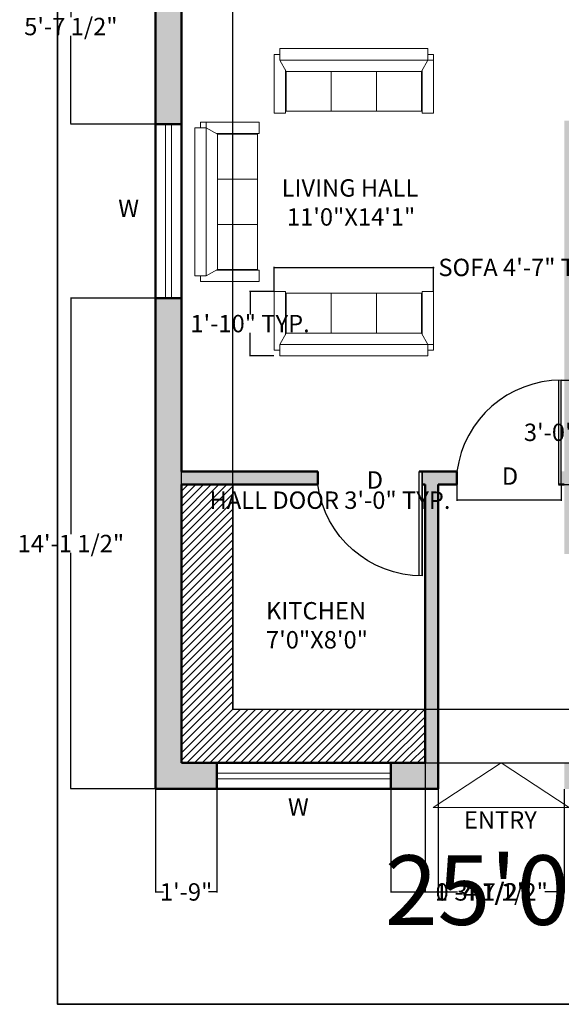
# Model space of a CAD drawing. Units: inches. Extents: x 125920 to 126336, y 366134 to 366735.
# Tile 1 of 6: x 125920 to 126106, y 366134 to 366473. Entities that reach past the tile are written whole.
import ezdxf

# ---------------------------------------------------------------- set-up
doc = ezdxf.new("R2010")
doc.units = ezdxf.units.IN
doc.header["$MEASUREMENT"] = 0
for name, color, linetype, lineweight in [('A-ANNO-DIMS', 2, 'Continuous', 18), ('A-ANNO-SYMB', 7, 'Continuous', 18), ('A-ANNO-TEXT', 7, 'Continuous', 18), ('A-ANNO-TTLB', 7, 'Continuous', 35), ('A-AREA-IDEN', 7, 'Continuous', 25), ('A-DOOR', 3, 'Continuous', 25), ('A-FLOR-FIXT', 8, 'Continuous', 25), ('A-FLOR-FIXT-PATT', 7, 'Continuous', 13), ('A-FURN', 8, 'Continuous', 18), ('A-GLAZ', 4, 'Continuous', 18), ('A-WALL', 7, 'Continuous', 50)]:
    doc.layers.add(name, color=color, linetype=linetype, lineweight=lineweight)
doc.layers.add('A-WALL-PATT', color=18, linetype='Continuous', lineweight=13, true_color=0x000000)
doc.styles.get("Standard").update_dxf_attribs({"font": 'arial.ttf'})
doc.dimstyles.get("Standard").update_dxf_attribs({"dimtxt": 6, "dimasz": 0.18, "dimexe": 0.18, "dimexo": 0.0625, "dimgap": 0.09, "dimtad": 0, "dimtih": 1, "dimtoh": 1, "dimdec": 1, "dimzin": 0, "dimdsep": 46, "dimlunit": 3, "dimtxsty": 'Standard', "dimcen": 0.09, "dimadec": 0, "dimazin": 0, "dimtfac": 1, "dimtdec": 1, "dimtofl": 0, "dimtmove": 0, "dimatfit": 3, "dimfxl": 1, "dimtolj": 1, "dimtzin": 0, "dimarcsym": 0})

# ---------------------------------------------------------------- blocks, each defined once
blk = doc.blocks.new('SOFA-3-SEAT')
for p, q in [((1.96, 55.04), (22.23, 55.04)), ((1.96, 55.04), (1.96, 53.08)), ((3.92, 55.04), (3.92, 1.96)), ((22.23, 51.12), (22.23, 55.04)), ((0, 53.08), (0, 1.96)), ((3.92, 53.08), (0, 53.08)), ((3.92, 53.08), (7.85, 50.88)), ((7.54, 51.12), (22.23, 51.12)), ((21.58, 50.87), (7.85, 50.87)), ((21.58, 35.3), (7.85, 35.3)), ((21.58, 19.74), (7.85, 19.74)), ((7.85, 4.17), (3.92, 1.96)), ((7.29, 3.92), (22.23, 3.92)), ((22.23, 3.92), (22.23, 0)), ((3.92, 1.96), (0, 1.96)), ((1.96, 1.96), (1.96, 0)), ((1.96, 0), (22.23, 0))]:
    blk.add_line(p, q)
blk.add_lwpolyline([(7.85, 50.88), (7.85, 4.17), (21.58, 4.17), (21.58, 50.87)])
blk = doc.blocks.new('WIN-60')
for p, q in [((0, 0), (0, 60)), ((3.5, 0), (3.5, 60)), ((5.5, 60), (5.5, 0)), ((9, 60), (9, 0))]:
    blk.add_line(p, q)
blk = doc.blocks.new('DOOR-36-WALL-4_5')
for p, q in [((0, 36), (0, 0)), ((0, 36), (1, 36)), ((1, 0), (1, 36))]:
    blk.add_line(p, q)
blk.add_arc((0, 36.32), 36.32, 270, 352.3719)
blk = doc.blocks.new('*D21')
at = {"layer": 'A-ANNO-DIMS', "color": 0, "lineweight": -2, "transparency": 16777216}
for p, q in [((126007.38, 366379.47), (126007.38, 366387.84)), ((126007.56, 366387.66), (126062.24, 366387.66)), ((126062.42, 366379.47), (126062.42, 366387.84)), ((126062.42, 366387.66), (126062.6, 366387.66))]:
    blk.add_line(p, q, dxfattribs=at)
at = {"layer": 'A-ANNO-DIMS', "color": 0, "transparency": 16777216}
for points in [[(126007.56, 366387.69), (126007.56, 366387.63), (126007.38, 366387.66)], [(126062.24, 366387.69), (126062.24, 366387.63), (126062.42, 366387.66)]]:
    blk.add_solid(points, dxfattribs=at)
at = {"layer": 'Defpoints', "color": 0, "transparency": 16777216}
for p in [(126062.42, 366387.66), (126007.38, 366379.4), (126062.42, 366379.4)]:
    blk.add_point(p, dxfattribs=at)
at = {"layer": 'A-ANNO-DIMS', "color": 0, "transparency": 16777216, "insert": (126093.54, 366387.66), "char_height": 6, "attachment_point": 5}
blk.add_mtext('\\A1;SOFA 4\'-7" TYP.', dxfattribs=at)
blk = doc.blocks.new('*D22')
at = {"layer": 'A-ANNO-DIMS', "color": 0, "lineweight": -2, "transparency": 16777216}
for p, q in [((126007.32, 366379.4), (125998.94, 366379.4)), ((125999.12, 366379.22), (125999.12, 366371.44)), ((125999.12, 366357.35), (125999.12, 366365.13)), ((126007.32, 366357.17), (125998.94, 366357.17))]:
    blk.add_line(p, q, dxfattribs=at)
at = {"layer": 'A-ANNO-DIMS', "color": 0, "transparency": 16777216}
for points in [[(125999.09, 366379.22), (125999.15, 366379.22), (125999.12, 366379.4)], [(125999.09, 366357.35), (125999.15, 366357.35), (125999.12, 366357.17)]]:
    blk.add_solid(points, dxfattribs=at)
at = {"layer": 'Defpoints', "color": 0, "transparency": 16777216}
for p in [(125999.12, 366379.4), (126007.38, 366379.4), (126007.38, 366357.17)]:
    blk.add_point(p, dxfattribs=at)
at = {"layer": 'A-ANNO-DIMS', "color": 0, "transparency": 16777216, "insert": (125999.12, 366368.29), "char_height": 6, "attachment_point": 5}
blk.add_mtext('\\A1;1\'-10" TYP.', dxfattribs=at)
blk = doc.blocks.new('*D23')
at = {"layer": 'A-ANNO-DIMS', "color": 0, "lineweight": -2, "transparency": 16777216}
for p, q in [((126070.47, 366312.73), (126070.47, 366307.21)), ((126106.47, 366312.73), (126106.47, 366307.21)), ((126070.47, 366307.39), (126070.29, 366307.39)), ((126106.29, 366307.39), (126070.65, 366307.39))]:
    blk.add_line(p, q, dxfattribs=at)
at = {"layer": 'A-ANNO-DIMS', "color": 0, "transparency": 16777216}
for points in [[(126070.65, 366307.42), (126070.65, 366307.36), (126070.47, 366307.39)], [(126106.29, 366307.42), (126106.29, 366307.36), (126106.47, 366307.39)]]:
    blk.add_solid(points, dxfattribs=at)
at = {"layer": 'Defpoints', "color": 0, "transparency": 16777216}
for p in [(126070.47, 366312.79), (126106.47, 366312.79), (126070.47, 366307.39)]:
    blk.add_point(p, dxfattribs=at)
at = {"layer": 'A-ANNO-DIMS', "color": 0, "transparency": 16777216, "insert": (126026.69, 366307.39), "char_height": 6, "attachment_point": 5}
blk.add_mtext('\\A1;HALL DOOR 3\'-0" TYP.', dxfattribs=at)
blk = doc.blocks.new('*D24')
at = {"layer": 'A-ANNO-DIMS', "color": 0, "lineweight": -2, "transparency": 16777216}
for p, q in [((126106.54, 366348.79), (126112.05, 366348.79)), ((126111.87, 366348.61), (126111.87, 366333.95)), ((126111.87, 366312.97), (126111.87, 366327.64)), ((126106.54, 366312.79), (126112.05, 366312.79))]:
    blk.add_line(p, q, dxfattribs=at)
at = {"layer": 'A-ANNO-DIMS', "color": 0, "transparency": 16777216}
for points in [[(126111.84, 366348.61), (126111.9, 366348.61), (126111.87, 366348.79)], [(126111.84, 366312.97), (126111.9, 366312.97), (126111.87, 366312.79)]]:
    blk.add_solid(points, dxfattribs=at)
at = {"layer": 'Defpoints', "color": 0, "transparency": 16777216}
for p in [(126106.47, 366348.79), (126106.47, 366312.79), (126111.87, 366312.79)]:
    blk.add_point(p, dxfattribs=at)
at = {"layer": 'A-ANNO-DIMS', "color": 0, "transparency": 16777216, "insert": (126111.87, 366330.79), "char_height": 6, "attachment_point": 5}
blk.add_mtext('\\A1;3\'-0" TYP.', dxfattribs=at)
blk = doc.blocks.new('*D29')
at = {"layer": 'A-ANNO-DIMS', "color": 0, "lineweight": -2, "transparency": 16777216}
for p, q in [((125966.41, 366377.07), (125937.14, 366377.07)), ((125937.32, 366376.89), (125937.32, 366295.63)), ((125937.32, 366207.97), (125937.32, 366289.24)), ((125966.41, 366207.79), (125937.14, 366207.79))]:
    blk.add_line(p, q, dxfattribs=at)
at = {"layer": 'A-ANNO-DIMS', "color": 0, "transparency": 16777216}
for points in [[(125937.29, 366376.89), (125937.35, 366376.89), (125937.32, 366377.07)], [(125937.29, 366207.97), (125937.35, 366207.97), (125937.32, 366207.79)]]:
    blk.add_solid(points, dxfattribs=at)
at = {"layer": 'Defpoints', "color": 0, "transparency": 16777216}
for p in [(125937.32, 366377.07), (125966.47, 366377.07), (125966.47, 366207.79)]:
    blk.add_point(p, dxfattribs=at)
at = {"layer": 'A-ANNO-DIMS', "color": 0, "transparency": 16777216, "insert": (125937.32, 366292.43), "char_height": 6, "attachment_point": 5}
blk.add_mtext('\\A1;14\'-1 1/2"', dxfattribs=at)
blk = doc.blocks.new('*D30')
at = {"layer": 'A-ANNO-DIMS', "color": 0, "lineweight": -2, "transparency": 16777216}
for p, q in [((125966.41, 366504.42), (125937.14, 366504.42)), ((125937.32, 366504.24), (125937.32, 366473.94)), ((125937.32, 366437.25), (125937.32, 366467.55)), ((125966.41, 366437.07), (125937.14, 366437.07))]:
    blk.add_line(p, q, dxfattribs=at)
at = {"layer": 'A-ANNO-DIMS', "color": 0, "transparency": 16777216}
for points in [[(125937.29, 366504.24), (125937.35, 366504.24), (125937.32, 366504.42)], [(125937.29, 366437.25), (125937.35, 366437.25), (125937.32, 366437.07)]]:
    blk.add_solid(points, dxfattribs=at)
at = {"layer": 'Defpoints', "color": 0, "transparency": 16777216}
for p in [(125937.32, 366504.42), (125966.47, 366504.42), (125966.47, 366437.07)]:
    blk.add_point(p, dxfattribs=at)
at = {"layer": 'A-ANNO-DIMS', "color": 0, "transparency": 16777216, "insert": (125937.32, 366470.74), "char_height": 6, "attachment_point": 5}
blk.add_mtext('\\A1;5\'-7 1/2"', dxfattribs=at)
blk = doc.blocks.new('*D36')
at = {"layer": 'A-ANNO-DIMS', "color": 0, "lineweight": -2, "transparency": 16777216}
for p, q in [((125966.47, 366207.73), (125966.47, 366172.1)), ((125987.64, 366207.73), (125987.64, 366172.1)), ((125966.65, 366172.28), (125969.28, 366172.28)), ((125987.46, 366172.28), (125984.84, 366172.28))]:
    blk.add_line(p, q, dxfattribs=at)
at = {"layer": 'A-ANNO-DIMS', "color": 0, "transparency": 16777216}
for points in [[(125966.65, 366172.31), (125966.65, 366172.25), (125966.47, 366172.28)], [(125987.46, 366172.31), (125987.46, 366172.25), (125987.64, 366172.28)]]:
    blk.add_solid(points, dxfattribs=at)
at = {"layer": 'Defpoints', "color": 0, "transparency": 16777216}
for p in [(125966.47, 366207.79), (125987.64, 366207.79), (125987.64, 366172.28)]:
    blk.add_point(p, dxfattribs=at)
at = {"layer": 'A-ANNO-DIMS', "color": 0, "transparency": 16777216, "insert": (125977.06, 366172.28), "char_height": 6, "attachment_point": 5}
blk.add_mtext('\\A1;1\'-9"', dxfattribs=at)
blk = doc.blocks.new('*D37')
at = {"layer": 'A-ANNO-DIMS', "color": 0, "lineweight": -2, "transparency": 16777216}
for p, q in [((126047.64, 366207.73), (126047.64, 366172.1)), ((126063.97, 366207.73), (126063.97, 366172.1)), ((126047.82, 366172.28), (126063.79, 366172.28)), ((126063.97, 366172.28), (126064.15, 366172.28))]:
    blk.add_line(p, q, dxfattribs=at)
at = {"layer": 'A-ANNO-DIMS', "color": 0, "transparency": 16777216}
for points in [[(126047.82, 366172.31), (126047.82, 366172.25), (126047.64, 366172.28)], [(126063.79, 366172.31), (126063.79, 366172.25), (126063.97, 366172.28)]]:
    blk.add_solid(points, dxfattribs=at)
at = {"layer": 'Defpoints', "color": 0, "transparency": 16777216}
for p in [(126047.64, 366207.79), (126063.97, 366207.79), (126063.97, 366172.28)]:
    blk.add_point(p, dxfattribs=at)
at = {"layer": 'A-ANNO-DIMS', "color": 0, "transparency": 16777216, "insert": (126078.93, 366172.28), "char_height": 6, "attachment_point": 5}
blk.add_mtext('\\A1;1\'-4 1/2"', dxfattribs=at)
blk = doc.blocks.new('*D38')
at = {"layer": 'A-ANNO-DIMS', "color": 0, "lineweight": -2, "transparency": 16777216}
for p, q in [((126063.97, 366207.73), (126063.97, 366172.1)), ((126107.47, 366207.73), (126107.47, 366172.1)), ((126064.15, 366172.28), (126070.67, 366172.28)), ((126107.29, 366172.28), (126100.78, 366172.28))]:
    blk.add_line(p, q, dxfattribs=at)
at = {"layer": 'A-ANNO-DIMS', "color": 0, "transparency": 16777216}
for points in [[(126064.15, 366172.31), (126064.15, 366172.25), (126063.97, 366172.28)], [(126107.29, 366172.31), (126107.29, 366172.25), (126107.47, 366172.28)]]:
    blk.add_solid(points, dxfattribs=at)
at = {"layer": 'Defpoints', "color": 0, "transparency": 16777216}
for p in [(126063.97, 366207.79), (126107.47, 366207.79), (126107.47, 366172.28)]:
    blk.add_point(p, dxfattribs=at)
at = {"layer": 'A-ANNO-DIMS', "color": 0, "transparency": 16777216, "insert": (126085.72, 366172.28), "char_height": 6, "attachment_point": 5}
blk.add_mtext('\\A1;3\'-7 1/2"', dxfattribs=at)
blk = doc.blocks.new('*D45')
at = {"layer": 'A-ANNO-DIMS', "color": 0, "lineweight": -2, "transparency": 16777216}
for p, q in [((125975.47, 366216.86), (125975.47, 366718.12)), ((125975.65, 366717.94), (125992.98, 366717.94)), ((125993.16, 366235.36), (125993.16, 366718.12)), ((125993.16, 366717.94), (125993.34, 366717.94))]:
    blk.add_line(p, q, dxfattribs=at)
at = {"layer": 'A-ANNO-DIMS', "color": 0, "transparency": 16777216}
for points in [[(125975.65, 366717.97), (125975.65, 366717.91), (125975.47, 366717.94)], [(125992.98, 366717.97), (125992.98, 366717.91), (125993.16, 366717.94)]]:
    blk.add_solid(points, dxfattribs=at)
at = {"layer": 'Defpoints', "color": 0, "transparency": 16777216}
for p in [(125993.16, 366717.94), (125993.16, 366235.3), (125975.47, 366216.79)]:
    blk.add_point(p, dxfattribs=at)
at = {"layer": 'A-ANNO-DIMS', "color": 0, "transparency": 16777216, "insert": (126008.11, 366717.94), "char_height": 6, "attachment_point": 5}
blk.add_mtext('\\A1;1\'-5 1/2"', dxfattribs=at)
blk = doc.blocks.new('*D46')
at = {"layer": 'A-ANNO-DIMS', "color": 0, "lineweight": -2, "transparency": 16777216}
for p, q in [((126059.54, 366235.3), (126295.8, 366235.3)), ((126295.62, 366235.12), (126295.62, 366229.24)), ((126295.62, 366216.97), (126295.62, 366222.85)), ((126059.54, 366216.79), (126295.8, 366216.79))]:
    blk.add_line(p, q, dxfattribs=at)
at = {"layer": 'A-ANNO-DIMS', "color": 0, "transparency": 16777216}
for points in [[(126295.59, 366235.12), (126295.65, 366235.12), (126295.62, 366235.3)], [(126295.59, 366216.97), (126295.65, 366216.97), (126295.62, 366216.79)]]:
    blk.add_solid(points, dxfattribs=at)
at = {"layer": 'Defpoints', "color": 0, "transparency": 16777216}
for p in [(126059.47, 366235.3), (126059.47, 366216.79), (126295.62, 366216.79)]:
    blk.add_point(p, dxfattribs=at)
at = {"layer": 'A-ANNO-DIMS', "color": 0, "transparency": 16777216, "insert": (126295.62, 366226.05), "char_height": 6, "attachment_point": 5}
blk.add_mtext('\\A1;1\'-6 1/2"', dxfattribs=at)
blk = doc.blocks.new('*D47')
at = {"layer": 'A-ANNO-DIMS', "color": 0, "lineweight": -2, "transparency": 16777216}
for p, q in [((126059.47, 366312.73), (126059.47, 366172.1)), ((126063.97, 366312.73), (126063.97, 366172.1)), ((126059.65, 366172.28), (126063.79, 366172.28)), ((126063.97, 366172.28), (126064.15, 366172.28))]:
    blk.add_line(p, q, dxfattribs=at)
at = {"layer": 'A-ANNO-DIMS', "color": 0, "transparency": 16777216}
for points in [[(126059.65, 366172.31), (126059.65, 366172.25), (126059.47, 366172.28)], [(126063.79, 366172.31), (126063.79, 366172.25), (126063.97, 366172.28)]]:
    blk.add_solid(points, dxfattribs=at)
at = {"layer": 'Defpoints', "color": 0, "transparency": 16777216}
for p in [(126059.47, 366312.79), (126063.97, 366312.79), (126063.97, 366172.28)]:
    blk.add_point(p, dxfattribs=at)
at = {"layer": 'A-ANNO-DIMS', "color": 0, "transparency": 16777216, "insert": (126079.21, 366172.28), "char_height": 6, "attachment_point": 5}
blk.add_mtext('\\A1;0\'-4 1/2"', dxfattribs=at)

msp = doc.modelspace()

# ---------------------------------------------------------------- hatches: boundary and pattern name
at = {"layer": 'A-FLOR-FIXT-PATT'}
h = msp.add_hatch(dxfattribs=at)
h.set_pattern_fill('ANSI31', color=256, scale=15)
h.paths.add_polyline_path([(125993.16, 366312.79), (125975.47, 366312.79), (125975.47, 366216.79), (126059.47, 366216.79), (126059.47, 366235.3), (125993.16, 366235.3)])
at = {"layer": 'A-WALL-PATT'}
h = msp.add_hatch(color=256, dxfattribs=at)
h.dxf.hatch_style = 1
h.paths.add_polyline_path([(126266.47, 366688.79), (125966.47, 366688.79), (125966.47, 366649.55), (125975.47, 366649.55), (125975.47, 366679.79), (126107.47, 366679.79), (126107.47, 366547.79), (126106.47, 366547.79), (126106.47, 366538.79), (126107.47, 366538.79), (126117.47, 366538.79), (126117.47, 366547.79), (126116.47, 366547.79), (126116.47, 366679.79), (126257.47, 366679.79), (126257.47, 366648.33), (126266.47, 366648.33)])
h.paths.add_polyline_path([(126070.47, 366547.79), (125975.47, 366547.79), (125975.47, 366589.55), (125966.47, 366589.55), (125966.47, 366528.42), (125975.47, 366528.42), (125975.47, 366538.79), (126059.47, 366538.79), (126059.47, 366515.79), (126063.97, 366515.79), (126063.97, 366538.79), (126070.47, 366538.79)])
h.paths.add_polyline_path([(125975.47, 366486.29), (126063.97, 366486.29), (126063.97, 366491.79), (126059.47, 366491.79), (126059.47, 366490.79), (125975.47, 366490.79), (125975.47, 366504.42), (125966.47, 366504.42), (125966.47, 366437.07), (125975.47, 366437.07)])
h.paths.add_polyline_path([(125975.47, 366312.79), (126022.47, 366312.79), (126022.47, 366317.29), (125975.47, 366317.29), (125975.47, 366377.07), (125966.47, 366377.07), (125966.47, 366207.79), (125987.64, 366207.79), (125987.64, 366216.79), (125975.47, 366216.79)])
h.paths.add_polyline_path([(126063.97, 366216.79), (126063.97, 366312.79), (126070.47, 366312.79), (126070.47, 366317.29), (126058.47, 366317.29), (126058.47, 366312.79), (126059.47, 366312.79), (126059.47, 366216.79), (126047.64, 366216.79), (126047.64, 366207.79), (126063.97, 366207.79)])
h.paths.add_polyline_path([(126221.47, 366216.79), (126116.47, 366216.79), (126107.47, 366216.79), (126107.47, 366207.79), (126221.47, 366207.79)])
h.paths.add_polyline_path([(126266.47, 366336.48), (126257.47, 366336.48), (126257.47, 366297.79), (126174.23, 366297.79), (126174.23, 366288.79), (126257.47, 366288.79), (126257.47, 366207.79), (126266.47, 366207.79)])
h.paths.add_polyline_path([(126138.23, 366297.79), (126116.47, 366297.79), (126116.47, 366433.79), (126117.47, 366433.79), (126117.47, 366438.29), (126116.47, 366438.29), (126107.47, 366438.29), (126107.47, 366317.29), (126106.47, 366317.29), (126106.47, 366312.79), (126107.47, 366312.79), (126107.47, 366288.79), (126116.47, 366288.79), (126138.23, 366288.79)])
h.paths.add_polyline_path([(126266.47, 366449.1), (126257.47, 366449.1), (126257.47, 366438.29), (126256.47, 366438.29), (126256.47, 366433.79), (126257.47, 366433.79), (126257.47, 366396.48), (126266.47, 366396.48)])
h.paths.add_polyline_path([(126232.47, 366438.29), (126180.47, 366438.29), (126180.47, 366486.29), (126257.47, 366486.29), (126257.47, 366473.1), (126266.47, 366473.1), (126266.47, 366504.78), (126257.47, 366504.78), (126257.47, 366490.79), (126180.47, 366490.79), (126180.47, 366538.79), (126232.47, 366538.79), (126232.47, 366547.79), (126153.47, 366547.79), (126153.47, 366538.79), (126175.97, 366538.79), (126175.97, 366438.29), (126153.47, 366438.29), (126153.47, 366433.79), (126232.47, 366433.79)])
h.paths.add_polyline_path([(126266.47, 366588.33), (126257.47, 366588.33), (126257.47, 366547.79), (126256.47, 366547.79), (126256.47, 366538.79), (126257.47, 366538.79), (126257.47, 366528.78), (126266.47, 366528.78)])

# ---------------------------------------------------------------- linework, layer by layer
at = {"layer": 'A-ANNO-SYMB'}
for p, q in [((126085.72, 366216.79), (126062.3, 366201.43)), ((126085.72, 366216.79), (126109.15, 366201.43)), ((126062.3, 366201.43), (126109.15, 366201.43))]:
    msp.add_line(p, q, dxfattribs=at)
at = {"layer": 'A-ANNO-TTLB'}
msp.add_lwpolyline([(125932.73, 366735.48), (126336.24, 366735.48), (126336.24, 366133.52), (125932.73, 366133.52)], close=True, dxfattribs=at)
at = {"layer": 'A-DOOR'}
for p in [(126059.47, 366317.29), (126058.47, 366281.29)]:
    msp.add_line(p, (126058.47, 366317.29), dxfattribs=at)
at = {"layer": 'A-FLOR-FIXT'}
for p, q in [((125993.16, 366312.79), (125993.16, 366235.3)), ((125993.16, 366235.3), (126059.47, 366235.3))]:
    msp.add_line(p, q, dxfattribs=at)
at = {"layer": 'A-WALL'}
for p, q in [((125966.47, 366688.79), (125966.47, 366207.79)), ((125975.47, 366486.29), (125975.47, 366317.29)), ((125966.47, 366437.07), (125975.47, 366437.07)), ((125975.47, 366377.07), (125966.47, 366377.07)), ((125975.47, 366317.29), (126022.47, 366317.29)), ((126022.47, 366317.29), (126022.47, 366312.79)), ((126057.47, 366317.29), (126070.47, 366317.29)), ((126070.47, 366312.79), (126070.47, 366317.29)), ((125975.47, 366312.79), (126022.47, 366312.79)), ((125975.47, 366312.79), (125975.47, 366216.79)), ((126058.47, 366312.79), (126059.47, 366312.79)), ((126059.47, 366312.79), (126059.47, 366216.79)), ((126063.97, 366312.79), (126063.97, 366216.79)), ((126063.97, 366312.79), (126070.47, 366312.79)), ((126105.47, 366312.79), (126107.47, 366312.79)), ((125975.47, 366216.79), (126059.47, 366216.79)), ((125987.64, 366216.79), (125987.64, 366207.79)), ((126047.64, 366207.79), (126047.64, 366216.79)), ((126063.97, 366216.79), (126063.97, 366207.79)), ((125966.47, 366207.79), (126063.97, 366207.79))]:
    msp.add_line(p, q, dxfattribs=at)

# ---------------------------------------------------------------- block references
at = {"layer": 'A-DOOR', "rotation": 180}
msp.add_blockref('DOOR-36-WALL-4_5', (126106.47, 366348.79), dxfattribs=at)
at = {"layer": 'A-DOOR', "extrusion": (0, 0, -1), "zscale": -1}
msp.add_blockref('DOOR-36-WALL-4_5', (-126058.47, 366281.29), dxfattribs=at)
at = {"layer": 'A-FURN', "rotation": 269.9999999993723}
msp.add_blockref('SOFA-3-SEAT', (126007.38, 366463.11), dxfattribs=at)
at = {"layer": 'A-FURN'}
msp.add_blockref('SOFA-3-SEAT', (125980.09, 366382.77), dxfattribs=at)
at = {"layer": 'A-FURN', "extrusion": (0, 0, -1), "zscale": -1, "rotation": 90.00000000006386}
msp.add_blockref('SOFA-3-SEAT', (-126007.38, 366357.17), dxfattribs=at)
at = {"layer": 'A-GLAZ'}
msp.add_blockref('WIN-60', (125966.47, 366377.07), dxfattribs=at)
at = {"layer": 'A-GLAZ', "rotation": 269.9999999998913}
msp.add_blockref('WIN-60', (125987.64, 366216.79), dxfattribs=at)

# ---------------------------------------------------------------- texts
at = {"layer": 'A-ANNO-TEXT', "char_height": 6, "attachment_point": 1}
for s, width, insert in [('W', 14.507, (125953.64, 366411.08)), ('D', 9.6923, (126039.35, 366317.35)), ('D', 9.6923, (126085.96, 366318.69)), ('W', 14.507, (126012.18, 366204.61)), ('ENTRY', 32.1345, (126072.87, 366200.1))]:
    msp.add_mtext_dynamic_manual_height_columns(s, width=width, gutter_width=30, heights=[0], dxfattribs=dict(at, insert=insert))
at = {"layer": 'A-ANNO-TTLB', "insert": (126045.63, 366184.9), "char_height": 24, "attachment_point": 1}
msp.add_mtext_dynamic_manual_height_columns('25\'0"X40\'0"', width=154.5965, gutter_width=30, heights=[0], dxfattribs=at)
at = {"layer": 'A-AREA-IDEN', "char_height": 6, "attachment_point": 1}
for s, width, insert in [('LIVING HALL\\P 11\'0"X14\'1"', 55.4081, (126010.01, 366418.08)), ('KITCHEN\\P7\'0"X8\'0"', 44.5323, (126004.61, 366272.24))]:
    msp.add_mtext_dynamic_manual_height_columns(s, width=width, gutter_width=30, heights=[0], dxfattribs=dict(at, insert=insert))

# ---------------------------------------------------------------- dimensions: what is measured, and where the dimension line sits
at = {"layer": 'A-ANNO-DIMS'}
for base, p1, p2, picture, middle in [((125993.16, 366717.94), (125975.47, 366216.79), (125993.16, 366235.3), '*D45', (126008.11, 366717.94)), ((126063.97, 366172.28), (126059.47, 366312.79), (126063.97, 366312.79), '*D47', (126079.21, 366172.28)), ((125987.64, 366172.28), (125966.47, 366207.79), (125987.64, 366207.79), '*D36', (125977.06, 366172.28)), ((126063.97, 366172.28), (126047.64, 366207.79), (126063.97, 366207.79), '*D37', (126078.93, 366172.28)), ((126107.47, 366172.28), (126063.97, 366207.79), (126107.47, 366207.79), '*D38', (126085.72, 366172.28))]:
    dim = msp.add_linear_dim(base=base, p1=p1, p2=p2, dimstyle='Standard', override={"dimdec": 1, "dimlfac": 1, "dimrnd": 0, "dimzin": 1, "dimdsep": 46, "dimlunit": 4, "dimfrac": 2}, dxfattribs=at)
    dim.commit()
    dim.dimension.update_dxf_attribs({"geometry": picture, "text_midpoint": middle})
for base, p1, p2, picture, middle in [((125937.3231, 366504.4154), (125966.4731, 366437.0722), (125966.4731, 366504.4154), '*D30', (125937.3231, 366470.7438)), ((125937.32, 366377.07), (125966.47, 366207.79), (125966.47, 366377.07), '*D29', (125937.32, 366292.43)), ((126295.62, 366216.79), (126059.47, 366235.3), (126059.47, 366216.79), '*D46', (126295.62, 366226.05))]:
    dim = msp.add_linear_dim(base=base, p1=p1, p2=p2, angle=90, dimstyle='Standard', override={"dimdec": 1, "dimlfac": 1, "dimrnd": 0, "dimzin": 1, "dimdsep": 46, "dimlunit": 4, "dimfrac": 2}, dxfattribs=at)
    dim.commit()
    dim.dimension.update_dxf_attribs({"geometry": picture, "text_midpoint": middle})
dim = msp.add_linear_dim(base=(126062.42, 366387.66), p1=(126007.38, 366379.4), p2=(126062.42, 366379.4), text='SOFA <> TYP.', dimstyle='Standard', override={"dimdec": 1, "dimlfac": 1, "dimrnd": 0, "dimzin": 1, "dimdsep": 46, "dimlunit": 4, "dimfrac": 2}, dxfattribs=at)
dim.commit()
dim.dimension.update_dxf_attribs({"geometry": '*D21', "text_midpoint": (126093.54, 366387.66)})
for base, p1, p2, angle, text, picture, middle in [((125999.12, 366379.4), (126007.38, 366357.17), (126007.38, 366379.4), 90, '<> TYP.', '*D22', (125999.12, 366368.29)), ((126111.87, 366312.79), (126106.47, 366348.79), (126106.47, 366312.79), 270, '<> TYP.', '*D24', (126111.87, 366330.79)), ((126070.47, 366307.39), (126106.47, 366312.79), (126070.47, 366312.79), 180, 'HALL DOOR <> TYP.', '*D23', (126026.69, 366307.39))]:
    dim = msp.add_linear_dim(base=base, p1=p1, p2=p2, angle=angle, text=text, dimstyle='Standard', override={"dimdec": 1, "dimlfac": 1, "dimrnd": 0, "dimzin": 1, "dimdsep": 46, "dimlunit": 4, "dimfrac": 2}, dxfattribs=at)
    dim.commit()
    dim.dimension.update_dxf_attribs({"geometry": picture, "text_midpoint": middle})

doc.saveas('drawing.dxf')
